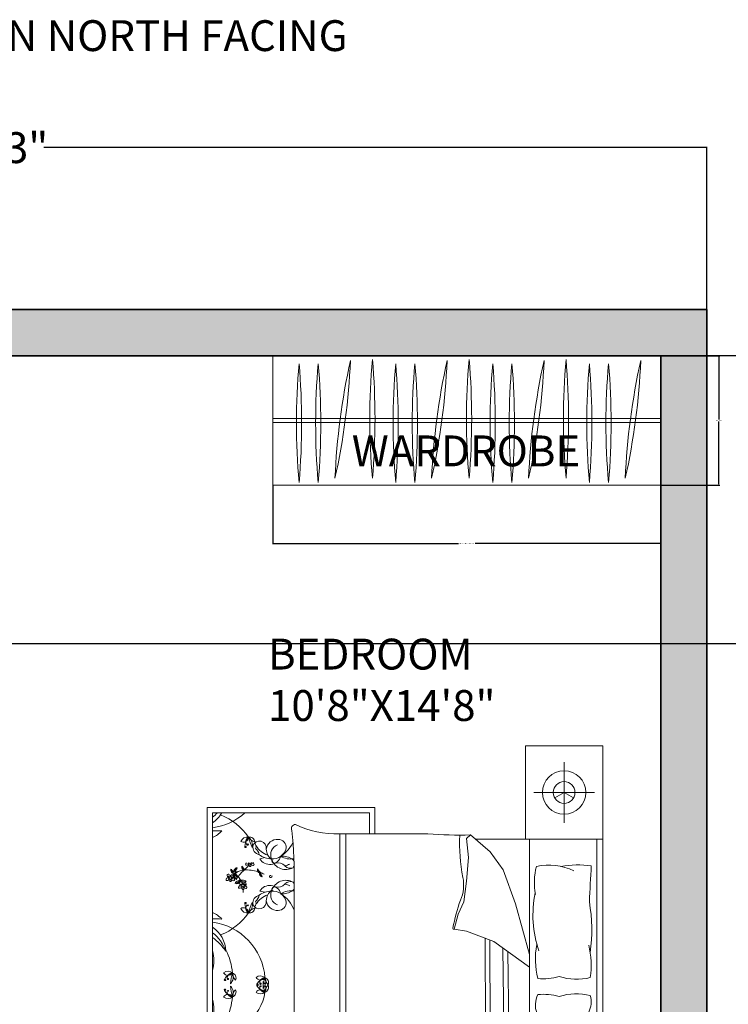
# Model space of a CAD drawing. Units: inches. Extents: x 37 to 706, y -568 to 110.
# Tile 21 of 24: x 224 to 362, y -84 to 108. Entities that reach past the tile are written whole.
import ezdxf

# ---------------------------------------------------------------- set-up
doc = ezdxf.new("R2010")
doc.units = ezdxf.units.IN
doc.header["$MEASUREMENT"] = 0
for name, color, linetype, lineweight in [('A-ANNO-DIMS', 2, 'Continuous', 18), ('A-ANNO-TEXT', 7, 'Continuous', 18), ('A-AREA-IDEN', 7, 'Continuous', 18), ('A-FLOR-CASE', 9, 'Continuous', 18), ('A-FURN', 8, 'Continuous', 13), ('A-WALL', 7, 'Continuous', 35), ('A-WALL-PATT', 252, 'Continuous', 13)]:
    doc.layers.add(name, color=color, linetype=linetype, lineweight=lineweight)
doc.styles.get("Standard").update_dxf_attribs({"font": 'arial.ttf'})
doc.dimstyles.get("Standard").update_dxf_attribs({"dimtxt": 0.18, "dimasz": 0.18, "dimexe": 0.18, "dimexo": 0.0625, "dimgap": 0.09, "dimtad": 0, "dimtih": 1, "dimtoh": 1, "dimdec": 0, "dimzin": 0, "dimdsep": 46, "dimlunit": 3, "dimtxsty": 'Standard', "dimcen": 0.09, "dimadec": 0, "dimazin": 0, "dimtfac": 1, "dimtdec": 0, "dimtofl": 0, "dimtmove": 0, "dimatfit": 3, "dimfxl": 1, "dimtolj": 1, "dimtzin": 0, "dimarcsym": 0})

# ---------------------------------------------------------------- blocks, each defined once
blk = doc.blocks.new('*D2')
at = {"layer": 'A-ANNO-DIMS', "color": 0, "lineweight": -2, "transparency": 16777216}
for p, q in [((78.96, 51.35), (78.96, 82.95)), ((79.14, 82.77), (208.01, 82.77)), ((357.78, 82.77), (228.91, 82.77)), ((357.96, 51.35), (357.96, 82.95))]:
    blk.add_line(p, q, dxfattribs=at)
at = {"layer": 'A-ANNO-DIMS', "color": 0, "transparency": 16777216}
for points in [[(79.14, 82.8), (79.14, 82.74), (78.96, 82.77)], [(357.78, 82.8), (357.78, 82.74), (357.96, 82.77)]]:
    blk.add_solid(points, dxfattribs=at)
at = {"layer": 'Defpoints', "color": 0, "transparency": 16777216}
for p in [(357.96, 82.77), (78.96, 51.29), (357.96, 51.29)]:
    blk.add_point(p, dxfattribs=at)
at = {"layer": 'A-ANNO-DIMS', "color": 0, "transparency": 16777216, "insert": (218.46, 82.77), "char_height": 6, "attachment_point": 5}
blk.add_mtext('\\A1;23\'-3"', dxfattribs=at)
blk = doc.blocks.new('WARDROBE-DOUBLE')
for p, q in [((75.49, 25.16), (0, 25.16)), ((0, 25.16), (0, 0)), ((75.49, 25.16), (75.49, 0)), ((75.49, 13), (0, 13)), ((75.49, 12.16), (0, 12.16)), ((75.49, 0), (0, 0))]:
    blk.add_line(p, q)
for centre, start, end in [((137.01, 12.08), 175.0028, 184.9972), ((-126.78, 12.08), 355.0028, 4.9972), ((140.74, 12.08), 175.0028, 184.9972), ((-123.05, 12.08), 355.0028, 4.9972), ((-117.16, 29.99), 347.508, 357.5023), ((144.38, -4.42), 167.508, 177.5023), ((151.29, 12.89), 175.0028, 184.9972), ((-112.5, 12.89), 355.0028, 4.9972), ((155.82, 12.08), 175.0028, 184.9972), ((-107.97, 12.08), 355.0028, 4.9972), ((159.55, 12.08), 175.0028, 184.9972), ((-104.24, 12.08), 355.0028, 4.9972), ((-98.35, 29.99), 347.508, 357.5023), ((163.19, -4.42), 167.508, 177.5023), ((170.1, 12.89), 175.0028, 184.9972), ((-93.69, 12.89), 355.0028, 4.9972), ((174.7, 12.08), 175.0028, 184.9972), ((-89.09, 12.08), 355.0028, 4.9972), ((178.43, 12.08), 175.0028, 184.9972), ((-85.36, 12.08), 355.0028, 4.9972), ((182.06, -4.42), 167.508, 177.5023), ((-79.47, 29.99), 347.508, 357.5023), ((188.97, 12.89), 175.0028, 184.9972), ((-74.82, 12.89), 355.0028, 4.9972), ((193.51, 12.08), 175.0028, 184.9972), ((-70.28, 12.08), 355.0028, 4.9972), ((197.24, 12.08), 175.0028, 184.9972), ((-66.55, 12.08), 355.0028, 4.9972), ((200.87, -4.42), 167.508, 177.5023), ((-60.66, 29.99), 347.508, 357.5023)]:
    blk.add_arc(centre, 132.4, start, end)
blk = doc.blocks.new('BED-DOUBLE-WITH-NIGHTSTANDS')
for p, q in [((77.02, 90.57), (77.02, 0)), ((69.47, 75.59), (69.47, 87.43)), ((63.56, 81.51), (75.39, 81.51)), ((0, 78.61), (32.62, 78.61)), ((0, 12.59), (0, 78.61)), ((32.62, 78.61), (32.62, 73.49)), ((1.05, 77.56), (1.05, 13.64)), ((31.58, 77.56), (1.05, 77.56)), ((31.58, 73.49), (31.58, 77.56)), ((25.85, 17.62), (25.85, 73.5)), ((26.98, 17.7), (26.98, 73.5)), ((50.48, 72.53), (51.22, 73.26)), ((51.22, 73.26), (55.07, 69.96)), ((50.85, 68.86), (50.48, 72.53)), ((77.02, 72.45), (52.16, 72.45)), ((62.71, 72.45), (62.71, 18.11)), ((75.86, 18.11), (75.86, 72.45)), ((55.07, 69.96), (57.63, 66.48)), ((10.23, 68.64), (11.25, 68.84)), ((50.48, 64.28), (50.85, 68.86)), ((57.63, 66.48), (60.02, 59.87)), ((16.95, 26.9), (16.95, 63.67)), ((49.93, 60.24), (50.48, 64.28)), ((10.23, 62.31), (11.25, 62.11)), ((48.83, 57.86), (49.93, 60.24)), ((60.02, 59.87), (62.71, 50)), ((48.1, 54.92), (48.83, 57.86)), ((50.48, 54.55), (48.1, 54.92)), ((55.8, 52.54), (50.48, 54.55)), ((54.24, 18.43), (54.09, 53.18)), ((55.17, 18.44), (55.03, 52.83)), ((62.71, 47.57), (55.8, 52.54)), ((58.02, 18.39), (57.55, 51.28)), ((58.95, 18.36), (58.49, 50.6)), ((10.23, 28.89), (11.25, 29.09)), ((10.23, 22.56), (11.25, 22.36)), ((31.58, 13.64), (31.58, 17.63)), ((32.62, 17.61), (32.62, 12.59)), ((1.05, 13.64), (31.58, 13.64)), ((69.47, 14.97), (69.47, 3.14)), ((32.62, 12.59), (0, 12.59))]:
    blk.add_line(p, q)
for points in [[(61.93, 72.45), (61.93, 90.57), (77.02, 90.57)], [(69.47, 81.51), (67.64, 80.45)], [(69.47, 81.51), (71.3, 80.45)], [(77.02, 18.11), (61.93, 18.11), (61.93, 0), (77.02, 0)], [(69.47, 9.06), (67.64, 10.11)], [(69.47, 9.06), (71.3, 10.11)]]:
    blk.add_lwpolyline(points)
for points in [[(42.92, 73.45, 0.001242), (25.74, 73.5, -0.127202), (17.18, 75.31)], [(74.76, 67.25, 0.074897), (68.85, 67.14, -0.472817)], [(68.52, 45.71, 0.14099), (74.55, 45.53, 0.235245)], [(68.52, 41.84, -0.14099), (74.55, 42.02, -0.235245)], [(74.76, 23.32, -0.074897), (68.85, 23.42, 0.472817)], [(27.69, 17.73, 0.056112), (22.71, 17.07, 0.095341), (17.91, 15.8)]]:
    blk.add_lwpolyline(points, format="xyb")
for centre, radius in [((69.47, 81.51), 4.23), ((69.47, 81.51), 2.11), ((4.52, 64.91), 0.231), ((6.95, 63.41), 0.231), ((6.95, 27.79), 0.231), ((4.52, 26.28), 0.231), ((69.47, 9.06), 4.23), ((69.47, 9.06), 2.11)]:
    blk.add_circle(centre, radius)
for centre, radius, start, end in [((-3.2, 82.51), 7.18, 306.3036, 316.4814), ((-2.13, 80.43), 5.76, 303.4617, 330.1116), ((-0.54, 86.37), 11.83, 277.745, 311.8856), ((-1.71, 66.13), 11.83, 34.3865, 68.5908), ((17.23, 74.48), 0.836, 93.98, 207.3412), ((-0.79, 77.21), 4.81, 292.5547, 318.9546), ((1.79, 90.38), 16.36, 267.4081, 273.6519), ((7.77, 71.53), 1.31, 77.7115, 159.0387), ((7.06, 72.84), 0.988, 238.4633, 358.2869), ((10.3, 70.85), 2.99, 138.8402, 177.9352), ((8.5, 71.96), 0.967, 117.6827, 223.7762), ((8.28, 71.86), 0.98, 2.9516, 103.728), ((16.12, 74.61), 8.27, 192.5173, 207.1824), ((6.95, 71.3), 1.87, 345.4653, 54.2343), ((9.77, 73.87), 2.02, 211.3827, 255.2969), ((-77.32, 64.75), 94.28, 359.3433, 5.6887), ((48.97, 156.3), 83.07, 265.8294, 271.553), ((83.29, 71.71), 34.18, 177.4519, 191.3392), ((7.46, 70.95), 0.147, 177.9352, 11.4834), ((7.53, 70.96), 0.0713, 11.4834, 127.9409), ((7.89, 71.38), 0.128, 223.7762, 159.7183), ((10.16, 70.71), 1.36, 350.264, 160.8688), ((10.57, 71.04), 1.7, 175.969, 254.3045), ((8.69, 70.99), 0.833, 333.9755, 53.2681), ((13.15, 73.4), 4.28, 211.2614, 251.7045), ((13.65, 70.21), 2.16, 84.9449, 172.8857), ((14.47, 69.36), 2.1, 111.5819, 201.4221), ((13.86, 70.84), 1.53, 354.4856, 91.0538), ((10.57, 74.83), 6.85, 303.6671, 333.2997), ((8.31, 69.21), 1.81, 6.1662, 51.5825), ((12.81, 73.44), 4.86, 236.2883, 266.5076), ((12.18, 69.76), 2.25, 209.9085, 343.1337), ((14.13, 70.59), 2.63, 182.3591, 234.0401), ((12.73, 71.31), 2.72, 265.2933, 346.921), ((16.28, 72.32), 3.75, 238.8218, 279.1554), ((14.65, 65.65), 3.49, 55.785, 94.7304), ((9.29, 67.11), 2.55, 178.3264, 187.1302), ((6.53, 66.75), 0.476, 11.3256, 64.4621), ((8.15, 67.44), 1.43, 190.2588, 210.656), ((1.34, 72.69), 8.6, 313.1541, 322.0459), ((7.66, 67.53), 0.177, 142.4737, 265.053), ((7.89, 67.56), 0.381, 127.7621, 169.0403), ((7.69, 67.89), 0.536, 265.053, 338.3618), ((8.4, 67.15), 0.7, 113.4276, 137.6104), ((8.32, 67.88), 0.231, 183.2768, 356.7232), ((8.49, 67.46), 0.377, 139.7889, 227.6792), ((8.37, 67.33), 0.199, 227.6792, 350.3487), ((7.6, 67.46), 0.755, 353.0852, 15.7171), ((8.1, 67.37), 0.477, 350.3487, 43.6538), ((8.98, 67.87), 0.555, 198.7263, 262.5032), ((8.54, 67.61), 0.22, 1.1081, 91.8675), ((8.68, 67.56), 0.385, 11.5637, 52.6358), ((8.95, 67.49), 0.178, 255.2356, 54.9248), ((13.13, 68.34), 0.562, 167.3041, 285.1471), ((14.65, 65.65), 3.49, 122.7011, 126.3445), ((15.31, 69.41), 2.89, 199.2822, 299.1751), ((13.76, 66), 1.86, 41.5653, 105.1471), ((14.78, 69.85), 2.6, 277.436, 299.9149), ((16.16, 68.13), 1.36, 221.5653, 293.8354), ((15.95, 67.67), 1.09, 30.0293, 52.325), ((15.95, 67.67), 1.09, 314.4517, 333.558), ((75.82, 64.02), 12.14, 165.1039, 191.0369), ((66.47, 55.71), 11.67, 65.1316, 101.7583), ((936.66, 17.33), 863.34, 176.68521, 177.14978), ((4.34, 65.38), 0.455, 157.4086, 261.4386), ((4.09, 65.4), 0.229, 58.0499, 135.6268), ((4.32, 65.26), 0.153, 172.906, 277.132), ((3.82, 64.98), 0.727, 14.7558, 58.0499), ((4.84, 65.17), 0.315, 36.1046, 181.4281), ((4.85, 66.4), 0.258, 124.3538, 214.3923), ((5.23, 66.36), 0.6, 190.3057, 287.1958), ((4.66, 65.42), 0.317, 270.0645, 331.1507), ((5.41, 66.58), 0.697, 176.9701, 248.2913), ((10.38, 70.25), 6.74, 212.6784, 216.3746), ((4.92, 65.2), 0.226, 263.7526, 41.7054), ((5.17, 66.41), 0.267, 216.3746, 291.7548), ((7.53, 62.67), 3.76, 124.0033, 132.4917), ((3.66, 62.2), 4.02, 63.7819, 68.2913), ((5.81, 65.29), 0.639, 128.3208, 208.8162), ((5.81, 66.23), 0.6, 122.8155, 187.3992), ((5.34, 65.98), 0.201, 289.3605, 111.7548), ((5.49, 65.98), 0.201, 221.8703, 44.2646), ((6.41, 65.39), 1.05, 157.2305, 229.0635), ((6.07, 66.15), 0.697, 109.4799, 177.6828), ((6.05, 65.74), 0.619, 174.4544, 220.6188), ((2.53, 62.29), 4.51, 30.544, 49.818), ((5.7, 66.59), 0.258, 56.8636, 146.9021), ((5.83, 66.31), 0.267, 148.8844, 224.2646), ((5.02, 64.86), 0.744, 340.0041, 40.6188), ((11.37, 62.96), 6.74, 145.1882, 148.8844), ((7.53, 62.67), 3.76, 94.756, 119.2041), ((15.54, 57.26), 12.37, 132.2412, 142.1744), ((7.19, 66.85), 0.435, 188.3432, 274.2869), ((7.57, 67.09), 0.759, 210.656, 242.6341), ((8.14, 67.75), 1.46, 218.2101, 226.3071), ((7.07, 66.52), 0.185, 325.7657, 67.4417), ((7.72, 58.94), 7.5, 73.5842, 93.8277), ((12.34, 66.57), 2.55, 178.3264, 187.1302), ((9.58, 66.21), 0.476, 11.3256, 64.4621), ((11.19, 66.9), 1.43, 190.2588, 210.656), ((10.23, 66.31), 0.435, 188.3432, 274.2869), ((10.61, 66.55), 0.759, 210.656, 242.6341), ((11.19, 67.21), 1.46, 218.2101, 226.3071), ((10.11, 65.98), 0.185, 325.7657, 67.4417), ((10.63, 65.65), 0.435, 147.5332, 233.4768), ((11.02, 65.87), 0.759, 179.1859, 211.164), ((10.28, 65.7), 0.185, 354.3784, 96.0543), ((7.72, 58.94), 7.5, 63.0032, 69.8941), ((11.6, 66.22), 1.43, 211.164, 231.5612), ((11.85, 67.38), 2.55, 234.6898, 243.4936), ((11.87, 66.07), 1.46, 195.5129, 203.6099), ((10.23, 65.12), 0.476, 357.3579, 50.4944), ((12.28, 65.21), 0.175, 12.7051, 190.4384), ((12.38, 65.23), 0.284, 190.4384, 10.4136), ((3.86, 64.56), 0.177, 142.4737, 265.053), ((4.09, 64.6), 0.381, 61.2196, 169.0403), ((3.89, 64.92), 0.536, 265.053, 338.3618), ((4.6, 64.19), 0.7, 113.4276, 137.6104), ((4.69, 64.5), 0.377, 139.7889, 227.6792), ((4.57, 64.37), 0.199, 227.6792, 350.3487), ((3.8, 64.5), 0.755, 353.0852, 15.7171), ((4.29, 64.41), 0.477, 350.3487, 43.6538), ((5.18, 64.9), 0.555, 198.7263, 262.5032), ((4.93, 65.34), 0.363, 221.8413, 265.7877), ((4.74, 64.65), 0.22, 1.1081, 91.8675), ((4.88, 64.6), 0.385, 11.5637, 86.365), ((5.15, 64.53), 0.178, 255.2356, 54.9248), ((5.92, 65.34), 0.764, 207.7043, 254.3516), ((5.43, 64.9), 1.05, 270.278, 342.111), ((6.13, 63.58), 0.744, 98.7227, 159.3375), ((5.75, 64.54), 0.764, 244.9899, 291.6373), ((5.92, 64.93), 0.619, 278.7227, 324.8872), ((5.81, 64.43), 0.639, 290.5253, 358.5375), ((6.52, 63.09), 0.381, 61.2196, 169.0403), ((6.32, 63.41), 0.536, 265.053, 338.3618), ((6.77, 63.88), 0.455, 157.4086, 261.4386), ((6.52, 63.89), 0.229, 58.0499, 135.6268), ((7.06, 64.61), 0.639, 182.8499, 266.1226), ((6.81, 65.06), 0.619, 231.7607, 277.9252), ((7.29, 65.17), 1.05, 214.5369, 286.3699), ((7.03, 62.68), 0.7, 113.4276, 137.6104), ((6.76, 63.75), 0.153, 172.906, 277.132), ((6.25, 63.47), 0.727, 14.7558, 58.0499), ((2.53, 62.29), 4.51, 23.0501, 23.8477), ((7.12, 62.99), 0.377, 139.7889, 227.6792), ((7, 63.71), 0.744, 37.3105, 97.9252), ((7.27, 63.66), 0.315, 36.1046, 181.4281), ((6.23, 62.99), 0.755, 353.0852, 15.7171), ((7.08, 64.73), 0.764, 265.0106, 311.658), ((6.72, 62.9), 0.477, 350.3487, 43.6538), ((7.61, 63.4), 0.555, 198.7263, 262.5032), ((7.09, 63.91), 0.317, 270.0645, 331.1507), ((7.36, 63.83), 0.363, 221.8413, 265.7877), ((7.17, 63.14), 0.22, 1.1081, 91.8675), ((7.36, 63.7), 0.226, 263.7526, 41.7054), ((7.31, 63.09), 0.385, 11.5637, 86.365), ((12.18, 61.19), 2.25, 16.8663, 150.0915), ((15.31, 61.54), 2.89, 60.8249, 160.7178), ((13.76, 64.95), 1.86, 254.8529, 318.4347), ((14.78, 61.1), 2.6, 60.0851, 82.564), ((16.16, 62.82), 1.36, 66.1646, 138.4347), ((15.95, 63.28), 1.09, 23.229, 45.5483), ((42.55, 63.54), 7.37, 336.2616, 11.3392), ((6.29, 63.06), 0.177, 142.4737, 265.053), ((7, 62.86), 0.199, 227.6792, 350.3487), ((2.53, 62.29), 4.51, 357.1071, 4.7585), ((7.58, 63.02), 0.178, 255.2356, 54.9248), ((10.57, 59.91), 1.7, 105.6955, 184.031), ((8.31, 61.74), 1.81, 308.4175, 353.8338), ((13.15, 57.54), 4.28, 108.2955, 148.7386), ((12.81, 57.5), 4.86, 93.4924, 123.7117), ((14.13, 60.36), 2.63, 125.9599, 177.6409), ((14.47, 61.59), 2.1, 158.5779, 248.4181), ((12.73, 59.64), 2.72, 13.079, 94.7067), ((13.13, 62.61), 0.562, 74.8529, 192.6959), ((14.65, 65.3), 3.49, 233.6555, 237.2989), ((16.28, 58.63), 3.75, 79.7133, 121.1782), ((14.65, 65.3), 3.49, 265.2696, 304.215), ((10.57, 56.11), 6.85, 21.4941, 56.3329), ((15.95, 63.28), 1.09, 307.675, 336.7144), ((84.45, 57.63), 21.05, 168.0397, 199.2615), ((7.46, 60), 0.147, 348.5166, 182.0648), ((10.3, 60.1), 2.99, 182.0648, 221.1598), ((7.53, 59.98), 0.0713, 232.0591, 348.5166), ((8.5, 58.99), 0.967, 136.2238, 242.3173), ((7.94, 59.56), 0.0771, 200.2667, 136.2271), ((6.95, 59.65), 1.87, 305.7657, 14.5347), ((16.12, 56.34), 8.27, 152.8176, 167.4827), ((10.16, 60.24), 1.36, 199.1312, 9.736), ((8.69, 59.96), 0.833, 306.7319, 26.0245), ((13.65, 60.74), 2.16, 187.1143, 275.0551), ((13.86, 60.11), 1.53, 268.9462, 5.5144), ((82.33, 48.63), 35.12, 160.1194, 169.3383), ((41.99, 54.84), 32.85, 352.2196, 9.497), ((-0.79, 53.74), 4.81, 41.0454, 67.4453), ((-1.71, 64.81), 11.83, 291.4092, 325.6135), ((7.06, 58.1), 0.988, 1.7131, 121.5367), ((7.77, 59.41), 1.31, 200.9613, 282.2885), ((8.28, 59.09), 0.98, 256.272, 357.0484), ((9.77, 57.08), 2.02, 104.7031, 148.6173), ((1.79, 40.57), 16.36, 86.3481, 92.5919), ((-0.54, 44.58), 11.83, 4.4623, 82.255), ((-2.13, 50.51), 5.76, 1.272, 56.5383), ((-3.2, 48.44), 7.18, 17.8504, 53.6964), ((48.03, 55.13), 0.219, 178.8623, 289.7536), ((-5.22, 44.66), 10.68, 34.0123, 54.053), ((79.85, 49.11), 15.97, 169.8617, 193.6238), ((58.59, 47.9), 16.14, 351.5249, 13.96), ((-5.17, 48.79), 6.5, 343.5431, 17.0202), ((-6.88, 45.48), 11.83, 4.4623, 27.4146), ((-8.52, 46.22), 9.62, 4.3787, 5.6357), ((-15.11, 41.15), 17.18, 19.7217, 19.9028), ((4.03, 45.43), 1.31, 47.7873, 129.1145), ((4.07, 46.92), 0.988, 208.5391, 328.3627), ((5.88, 43.58), 2.99, 108.9159, 148.011), ((4.87, 45.44), 0.967, 87.7585, 193.852), ((12.81, 43.93), 8.27, 162.593, 177.2582), ((3.21, 45.64), 1.87, 315.5411, 24.3101), ((6.93, 46.46), 2.02, 181.4585, 225.3727), ((4.64, 45.46), 0.98, 333.0274, 73.8037), ((3.47, 45.08), 0.147, 148.011, 341.5592), ((3.54, 45.06), 0.0713, 341.5592, 98.0167), ((4.06, 45.24), 0.128, 193.852, 129.9245), ((10.37, 44.53), 1.31, 47.7873, 129.1145), ((10.41, 46.02), 0.988, 208.5391, 328.3627), ((9.8, 44.18), 0.147, 148.011, 341.5592), ((9.8, 44), 0.147, 18.4408, 211.989), ((12.22, 42.67), 2.99, 108.9159, 148.011), ((9.88, 44.15), 0.0713, 341.5592, 98.0167), ((9.88, 44.03), 0.0713, 261.9833, 18.4408), ((11.21, 44.53), 0.967, 87.7585, 193.852), ((10.39, 44.33), 0.128, 193.852, 129.9245), ((9.54, 44.73), 1.87, 315.5411, 24.3101), ((19.14, 43.02), 8.27, 162.593, 177.2582), ((9.54, 43.45), 1.87, 335.6899, 44.4589), ((19.14, 45.16), 8.27, 182.7418, 197.407), ((10.97, 44.56), 0.98, 333.0274, 73.8037), ((13.27, 45.55), 2.02, 181.4585, 225.3727), ((10.97, 43.62), 0.98, 286.1963, 26.9726), ((13.27, 42.63), 2.02, 134.6273, 178.5415), ((65.49, 56.38), 11.1, 264.0129, 285.8293), ((2.19, 43.98), 9.15, 262.8636, 351.8197), ((4.07, 41.26), 0.988, 31.6373, 151.4609), ((3.47, 43.1), 0.147, 18.4408, 211.989), ((5.88, 44.6), 2.99, 211.989, 251.0841), ((3.54, 43.12), 0.0713, 261.9833, 18.4408), ((4.87, 42.74), 0.967, 166.148, 272.2415), ((4.11, 42.95), 0.0771, 230.1909, 166.0209), ((12.81, 44.25), 8.27, 182.7418, 197.407), ((3.21, 42.54), 1.87, 335.6899, 44.4589), ((6.93, 41.72), 2.02, 134.6273, 178.5415), ((4.64, 42.72), 0.98, 286.1963, 26.9726), ((10.41, 42.16), 0.988, 31.6373, 151.4609), ((10.37, 43.65), 1.31, 230.8855, 312.2127), ((12.22, 45.51), 2.99, 211.989, 251.0841), ((11.21, 43.65), 0.967, 166.148, 272.2415), ((10.44, 43.86), 0.0771, 230.1909, 166.0209), ((68.68, 40.17), 4.8, 155.0183, 198.5407), ((65.49, 31.16), 11.1, 74.1707, 95.9871), ((-5.17, 39.39), 6.5, 342.9798, 16.4569), ((-8.52, 41.96), 9.62, 354.3643, 355.6213), ((-15.11, 47.03), 17.18, 340.0972, 340.2783), ((4.03, 42.75), 1.31, 230.8855, 312.2127), ((-6.88, 42.69), 11.83, 332.5854, 355.5377), ((70.25, 40.78), 4.48, 333.3437, 16.1026), ((3.02, 42.8), 5.3, 248.117, 276.6195), ((1.55, 37.94), 2.12, 256.3898, 349.0739), ((1.84, 39.54), 2.68, 252.8609, 311.9049), ((-1.71, 26.39), 11.83, 34.3865, 68.5908), ((74.93, 31.78), 11.53, 153.8761, 196.1746), ((58.92, 34.06), 15.92, 346.3427, 11.1841), ((1.79, 50.63), 16.36, 267.4081, 273.6519), ((-0.79, 37.46), 4.81, 292.5547, 318.9546), ((7.77, 31.78), 1.31, 77.7115, 159.0387), ((7.06, 33.09), 0.988, 238.4633, 358.2869), ((10.3, 31.1), 2.99, 138.8402, 177.9352), ((8.5, 32.21), 0.967, 117.6827, 223.7762), ((8.28, 32.11), 0.98, 2.9516, 103.728), ((9.77, 34.12), 2.02, 211.3827, 255.2969), ((6.95, 31.55), 1.87, 345.4653, 54.2343), ((16.12, 34.86), 8.27, 192.5173, 207.1824), ((13.65, 30.46), 2.16, 84.9449, 172.8857), ((13.86, 31.09), 1.53, 354.4856, 91.0538), ((10.57, 35.08), 6.85, 303.6671, 338.5059), ((7.46, 31.2), 0.147, 177.9352, 11.4834), ((7.53, 31.21), 0.0713, 11.4834, 127.9409), ((7.89, 31.63), 0.128, 223.7762, 159.7183), ((10.16, 30.96), 1.36, 350.264, 160.8688), ((10.57, 31.29), 1.7, 175.969, 254.3045), ((8.69, 31.24), 0.833, 333.9755, 53.2681), ((8.31, 29.46), 1.81, 6.1662, 51.5825), ((13.15, 33.66), 4.28, 211.2614, 251.7045), ((14.13, 30.84), 2.63, 182.3591, 234.0401), ((14.47, 29.61), 2.1, 111.5819, 201.4221), ((12.73, 31.56), 2.72, 265.2933, 346.921), ((2.53, 28.91), 4.51, 355.2415, 2.8929), ((12.81, 33.7), 4.86, 236.2883, 266.5076), ((12.18, 30.01), 2.25, 209.9085, 343.1337), ((14.65, 25.9), 3.49, 122.7011, 126.3445), ((16.28, 32.57), 3.75, 238.8218, 280.2867), ((14.65, 25.9), 3.49, 55.785, 94.7304), ((15.95, 27.92), 1.09, 23.2856, 52.325), ((75.82, 26.55), 12.14, 168.9631, 194.8961), ((936.66, 73.23), 863.34, 182.85022, 183.31479), ((3.86, 26.63), 0.177, 94.947, 217.5263), ((3.89, 26.28), 0.536, 21.6382, 94.947), ((4.69, 26.7), 0.377, 132.3208, 220.2111), ((4.57, 26.83), 0.199, 9.6513, 132.3208), ((4.29, 26.79), 0.477, 316.3462, 9.6513), ((5.18, 26.29), 0.555, 97.4968, 161.2737), ((5.15, 26.67), 0.178, 305.0752, 104.7644), ((5.75, 26.66), 0.764, 68.3627, 115.0101), ((5.43, 26.3), 1.05, 17.889, 89.722), ((6.13, 27.61), 0.744, 200.6625, 261.2773), ((5.92, 26.27), 0.619, 35.1128, 81.2773), ((5.81, 26.77), 0.639, 1.4625, 69.4747), ((6.29, 28.14), 0.177, 94.947, 217.5263), ((6.52, 28.11), 0.381, 190.9597, 298.7804), ((6.32, 27.78), 0.536, 21.6382, 94.947), ((6.77, 27.32), 0.455, 98.5614, 202.5914), ((6.52, 27.31), 0.229, 224.3732, 301.9501), ((7.06, 26.59), 0.639, 93.8774, 177.1501), ((7.29, 26.03), 1.05, 73.6301, 145.4631), ((7.03, 28.52), 0.7, 222.3896, 246.5724), ((6.76, 27.45), 0.153, 82.868, 187.094), ((6.25, 27.73), 0.727, 301.9501, 345.2442), ((2.53, 28.91), 4.51, 336.1523, 336.9499), ((7.12, 28.21), 0.377, 132.3208, 220.2111), ((7, 28.34), 0.199, 9.6513, 132.3208), ((7, 27.49), 0.744, 262.0748, 322.6895), ((6.23, 28.2), 0.755, 344.2829, 6.9148), ((7.27, 27.54), 0.315, 178.5719, 323.8954), ((7.08, 26.46), 0.764, 48.342, 94.9894), ((6.72, 28.3), 0.477, 316.3462, 9.6513), ((7.61, 27.8), 0.555, 97.4968, 161.2737), ((7.36, 27.37), 0.363, 94.2123, 138.1587), ((7.09, 27.29), 0.317, 28.8493, 89.9355), ((7.17, 28.06), 0.22, 268.1325, 358.8919), ((7.31, 28.11), 0.385, 273.635, 348.4363), ((7.36, 27.5), 0.226, 318.2946, 96.2474), ((7.58, 28.18), 0.178, 305.0752, 104.7644), ((13.13, 28.59), 0.562, 167.3041, 285.1471), ((15.31, 29.66), 2.89, 199.2822, 299.1751), ((13.76, 26.25), 1.86, 41.5653, 105.1471), ((14.78, 30.1), 2.6, 277.436, 299.9149), ((16.16, 28.38), 1.36, 221.5653, 293.8354), ((-71.13, 24.12), 88.13, 355.2402, 1.8035), ((15.95, 27.92), 1.09, 314.4517, 336.7144), ((4.09, 26.6), 0.381, 190.9597, 298.7804), ((4.34, 25.81), 0.455, 98.5614, 202.5914), ((4.09, 25.8), 0.229, 224.3732, 301.9501), ((4.6, 27.01), 0.7, 222.3896, 246.5724), ((4.32, 25.94), 0.153, 82.868, 187.094), ((3.82, 26.22), 0.727, 301.9501, 345.2442), ((4.84, 26.03), 0.315, 178.5719, 323.8954), ((3.8, 26.7), 0.755, 344.2829, 6.9148), ((4.85, 24.8), 0.258, 145.6077, 235.6462), ((5.23, 24.83), 0.6, 72.8042, 169.6943), ((4.93, 25.86), 0.363, 94.2123, 138.1587), ((4.66, 25.78), 0.317, 28.8493, 89.9355), ((5.41, 24.62), 0.697, 111.7087, 183.0299), ((10.38, 20.95), 6.74, 143.6254, 147.3216), ((4.74, 26.55), 0.22, 268.1325, 358.8919), ((4.88, 26.6), 0.385, 273.635, 348.4363), ((4.92, 25.99), 0.226, 318.2946, 96.2474), ((5.17, 24.78), 0.267, 68.2452, 143.6254), ((7.53, 28.53), 3.76, 227.5083, 235.9967), ((3.66, 29), 4.02, 291.7087, 296.2181), ((5.81, 25.91), 0.639, 151.1838, 231.6792), ((5.81, 24.97), 0.6, 172.6008, 237.1845), ((5.92, 25.86), 0.764, 105.6484, 152.2957), ((5.34, 25.22), 0.201, 248.2452, 70.6395), ((6.41, 25.8), 1.05, 130.9365, 202.7695), ((5.49, 25.22), 0.201, 315.7354, 138.1297), ((6.07, 25.05), 0.697, 182.3172, 250.5201), ((6.05, 25.46), 0.619, 139.3812, 185.5456), ((2.53, 28.91), 4.51, 310.182, 329.456), ((5.83, 24.89), 0.267, 135.7354, 211.1156), ((5.02, 26.34), 0.744, 319.3812, 19.9959), ((7.53, 28.53), 3.76, 240.7959, 265.244), ((15.54, 33.94), 12.37, 217.8256, 227.7588), ((6.81, 26.14), 0.619, 82.0748, 128.2393), ((7.72, 32.26), 7.5, 266.1723, 286.4158), ((11.19, 24.3), 1.43, 149.344, 169.7412), ((12.34, 24.63), 2.55, 172.8698, 181.6736), ((10.23, 24.88), 0.435, 85.7131, 171.6568), ((10.61, 24.64), 0.759, 117.3659, 149.344), ((11.19, 23.99), 1.46, 133.6929, 141.7899), ((10.11, 25.21), 0.185, 292.5583, 34.2343), ((10.63, 25.55), 0.435, 126.5232, 212.4668), ((11.02, 25.33), 0.759, 148.836, 180.8141), ((10.28, 25.5), 0.185, 263.9457, 5.6216), ((7.72, 32.26), 7.5, 290.1059, 296.9968), ((11.6, 24.98), 1.43, 128.4388, 148.836), ((11.85, 23.82), 2.55, 116.5064, 125.3102), ((11.87, 25.13), 1.46, 156.3901, 164.4871), ((10.23, 26.08), 0.476, 309.5056, 2.6421), ((12.28, 25.98), 0.175, 169.5616, 347.2949), ((12.38, 25.96), 0.284, 349.5864, 169.5616), ((5.7, 24.61), 0.258, 213.0979, 303.1364), ((11.37, 28.24), 6.74, 211.1156, 214.8118), ((8.15, 23.76), 1.43, 149.344, 169.7412), ((9.29, 24.09), 2.55, 172.8698, 181.6736), ((6.53, 24.45), 0.476, 295.5379, 348.6744), ((7.19, 24.34), 0.435, 85.7131, 171.6568), ((7.57, 24.1), 0.759, 117.3659, 149.344), ((8.14, 23.45), 1.46, 133.6929, 141.7899), ((7.07, 24.67), 0.185, 292.5583, 34.2343), ((1.34, 18.5), 8.6, 37.9541, 46.8459), ((7.66, 23.67), 0.177, 94.947, 217.5263), ((7.89, 23.64), 0.381, 190.9597, 232.2379), ((7.69, 23.31), 0.536, 21.6382, 94.947), ((8.4, 24.05), 0.7, 222.3896, 246.5724), ((8.32, 23.32), 0.231, 3.2768, 176.7232), ((8.49, 23.74), 0.377, 132.3208, 220.2111), ((8.37, 23.87), 0.199, 9.6513, 132.3208), ((7.6, 23.73), 0.755, 344.2829, 6.9148), ((8.1, 23.82), 0.477, 316.3462, 9.6513), ((8.98, 23.33), 0.555, 97.4968, 161.2737), ((8.54, 23.59), 0.22, 268.1325, 358.8919), ((8.95, 23.71), 0.178, 305.0752, 104.7644), ((8.68, 23.64), 0.385, 307.3642, 348.4363), ((9.58, 24.98), 0.476, 295.5379, 348.6744), ((12.18, 21.44), 2.25, 16.8663, 150.0915), ((13.13, 22.86), 0.562, 74.8529, 192.6959), ((15.31, 21.79), 2.89, 60.8249, 160.7178), ((13.76, 25.2), 1.86, 254.8529, 318.4347), ((14.78, 21.35), 2.6, 60.0851, 82.564), ((16.16, 23.07), 1.36, 66.1646, 138.4347), ((15.95, 23.53), 1.09, 307.675, 342.5814), ((15.95, 23.53), 1.09, 16.6343, 45.5483), ((66.47, 34.85), 11.67, 258.2417, 294.8684), ((10.57, 20.16), 1.7, 105.6955, 184.031), ((8.31, 21.99), 1.81, 308.4175, 353.8338), ((13.15, 17.79), 4.28, 108.2955, 148.7386), ((12.81, 17.75), 4.86, 93.4924, 123.7117), ((14.13, 20.61), 2.63, 125.9599, 177.6409), ((14.47, 21.84), 2.1, 158.5779, 248.4181), ((12.73, 19.89), 2.72, 13.079, 94.7067), ((14.65, 25.55), 3.49, 233.6555, 237.2989), ((16.28, 18.88), 3.75, 79.249, 121.1782), ((14.65, 25.55), 3.49, 265.2696, 304.215), ((10.57, 16.37), 6.85, 23.6453, 56.3329), ((7.06, 18.36), 0.988, 1.7131, 121.5367), ((7.77, 19.67), 1.31, 200.9613, 282.2885), ((7.46, 20.25), 0.147, 348.5166, 182.0648), ((10.3, 20.35), 2.99, 182.0648, 221.1598), ((7.53, 20.24), 0.0713, 232.0591, 348.5166), ((8.5, 19.24), 0.967, 136.2238, 242.3173), ((7.94, 19.81), 0.0771, 200.2667, 136.2271), ((16.12, 16.59), 8.27, 152.8176, 167.4827), ((6.95, 19.9), 1.87, 305.7657, 14.5347), ((9.77, 17.33), 2.02, 104.7031, 148.6173), ((8.28, 19.34), 0.98, 256.272, 357.0484), ((10.16, 20.49), 1.36, 199.1312, 9.736), ((8.69, 20.21), 0.833, 306.7319, 26.0245), ((13.65, 20.99), 2.16, 187.1143, 275.0551), ((13.86, 20.36), 1.53, 268.9462, 5.5144), ((-0.79, 13.99), 4.81, 41.0454, 67.4453), ((-1.71, 25.06), 11.83, 291.4092, 325.6135), ((45.72, -193.78), 212.28, 89.1145, 94.8735), ((51.64, -144.24), 162.73, 86.1, 90.9282), ((1.79, 0.82), 16.36, 86.3481, 92.5919), ((-0.54, 4.83), 11.83, 48.1144, 82.255), ((-2.13, 10.76), 5.76, 29.8884, 56.5383), ((17.45, 16.48), 0.826, 156.5219, 303.8264), ((-3.2, 8.69), 7.18, 43.5186, 53.6964)]:
    blk.add_arc(centre, radius, start, end)
blk = doc.blocks.new('*D21')
at = {"layer": 'A-ANNO-DIMS', "color": 0, "lineweight": -2, "transparency": 16777216}
for p, q in [((273.47, 17.07), (273.47, 5.63)), ((348.96, 17.07), (348.96, 5.63)), ((273.65, 5.81), (309.59, 5.81)), ((348.78, 5.81), (312.84, 5.81))]:
    blk.add_line(p, q, dxfattribs=at)
at = {"layer": 'A-ANNO-DIMS', "color": 0, "transparency": 16777216}
for points in [[(273.65, 5.84), (273.65, 5.78), (273.47, 5.81)], [(348.78, 5.84), (348.78, 5.78), (348.96, 5.81)]]:
    blk.add_solid(points, dxfattribs=at)
at = {"layer": 'Defpoints', "color": 0, "transparency": 16777216}
for p in [(273.47, 17.13), (348.96, 17.13), (348.96, 5.81)]:
    blk.add_point(p, dxfattribs=at)
at = {"layer": 'A-ANNO-DIMS', "color": 0, "transparency": 16777216, "insert": (311.21, 5.81), "char_height": 0.18, "attachment_point": 5}
blk.add_mtext('\\A1;WARDROBE 6\'-3 1/2" TYP.', dxfattribs=at)
blk = doc.blocks.new('*D22')
at = {"layer": 'A-ANNO-DIMS', "color": 0, "lineweight": -2, "transparency": 16777216}
for p, q in [((349.02, 42.29), (360.46, 42.29)), ((360.28, 42.11), (360.28, 29.89)), ((360.28, 17.31), (360.28, 29.53)), ((349.02, 17.13), (360.46, 17.13))]:
    blk.add_line(p, q, dxfattribs=at)
at = {"layer": 'A-ANNO-DIMS', "color": 0, "transparency": 16777216}
for points in [[(360.25, 42.11), (360.31, 42.11), (360.28, 42.29)], [(360.25, 17.31), (360.31, 17.31), (360.28, 17.13)]]:
    blk.add_solid(points, dxfattribs=at)
at = {"layer": 'Defpoints', "color": 0, "transparency": 16777216}
for p in [(348.96, 42.29), (360.28, 42.29), (348.96, 17.13)]:
    blk.add_point(p, dxfattribs=at)
at = {"layer": 'A-ANNO-DIMS', "color": 0, "transparency": 16777216, "insert": (360.28, 29.71), "char_height": 0.18, "attachment_point": 5}
blk.add_mtext('\\A1;2\'-1" TYP.', dxfattribs=at)
blk = doc.blocks.new('*D42')
at = {"layer": 'A-ANNO-DIMS', "color": 0, "lineweight": -2, "transparency": 16777216}
for p, q in [((402.9, 42.29), (46.03, 42.29)), ((46.21, 42.11), (46.21, 14.47)), ((46.21, -13.53), (46.21, 14.11)), ((402.9, -13.71), (46.03, -13.71))]:
    blk.add_line(p, q, dxfattribs=at)
at = {"layer": 'A-ANNO-DIMS', "color": 0, "transparency": 16777216}
for points in [[(46.18, 42.11), (46.24, 42.11), (46.21, 42.29)], [(46.18, -13.53), (46.24, -13.53), (46.21, -13.71)]]:
    blk.add_solid(points, dxfattribs=at)
at = {"layer": 'Defpoints', "color": 0, "transparency": 16777216}
for p in [(402.96, 42.29), (46.21, -13.71), (402.96, -13.71)]:
    blk.add_point(p, dxfattribs=at)
at = {"layer": 'A-ANNO-DIMS', "color": 0, "transparency": 16777216, "insert": (46.21, 14.29), "char_height": 0.18, "attachment_point": 5}
blk.add_mtext('\\A1;4\'-8"', dxfattribs=at)

msp = doc.modelspace()

# ---------------------------------------------------------------- hatches: boundary and pattern name
at = {"layer": 'A-WALL-PATT'}
h = msp.add_hatch(color=256, dxfattribs=at)
h.dxf.hatch_style = 1
h.paths.add_polyline_path([(220.96, -351.71), (211.96, -351.71), (211.96, -513.71), (254.96, -513.71), (254.96, -504.71), (220.96, -504.71)], flags=17)
h.paths.add_polyline_path([(220.96, -294.71), (211.96, -294.71), (211.96, -303.71), (220.96, -303.71)], flags=17)
h.paths.add_polyline_path([(175.96, -294.71), (155.87, -294.71), (155.87, -303.71), (155.96, -303.71), (175.96, -303.71)], flags=17)
h.paths.add_polyline_path([(220.96, -16.71), (211.96, -16.71), (211.96, -142.71), (220.96, -142.71)], flags=17)
h.paths.add_polyline_path([(357.96, 51.29), (78.96, 51.29), (78.96, -513.71), (87.96, -513.71), (87.96, -303.71), (95.87, -303.71), (95.87, -294.71), (87.96, -294.71), (87.96, -142.71), (187.96, -142.71), (187.96, -133.71), (87.96, -133.71), (87.96, -25.71), (106.96, -25.71), (106.96, -16.71), (87.96, -16.71), (87.96, 42.29), (348.96, 42.29), (348.96, 17.13), (348.96, -133.71), (246.96, -133.71), (246.96, -142.71), (348.96, -142.71), (348.96, -294.71), (251.96, -294.71), (251.96, -303.71), (348.96, -303.71), (348.96, -351.71), (260.96, -351.71), (260.96, -329.71), (251.96, -329.71), (251.96, -360.71), (327.45, -360.71), (348.96, -360.71), (348.96, -504.71), (314.96, -504.71), (314.96, -513.71), (357.96, -513.71)])
h.paths.add_polyline_path([(416.96, -303.71), (402.96, -303.71), (402.96, -151.71), (478.96, -151.71), (478.96, -142.71), (402.96, -142.71), (402.96, -22.71), (409.96, -22.71), (409.96, -13.71), (402.96, -13.71), (402.96, 42.29), (663.96, 42.29), (663.96, -303.71), (566.96, -303.71), (566.96, -312.71), (663.96, -312.71), (663.96, -360.71), (575.96, -360.71), (575.96, -338.71), (566.96, -338.71), (566.96, -360.71), (566.96, -369.71), (642.45, -369.71), (663.96, -369.71), (663.96, -513.71), (629.96, -513.71), (629.96, -522.71), (672.96, -522.71), (672.96, 51.29), (393.96, 51.29), (393.96, -522.71), (402.96, -522.71), (402.96, -312.71), (416.96, -312.71)])
h.paths.add_polyline_path([(490.96, -303.71), (476.96, -303.71), (476.96, -312.71), (490.96, -312.71)], flags=17)
h.paths.add_polyline_path([(535.96, -303.71), (526.96, -303.71), (526.96, -312.71), (535.96, -312.71)], flags=17)
h.paths.add_polyline_path([(535.96, -369.71), (526.96, -369.71), (526.96, -522.71), (569.96, -522.71), (569.96, -513.71), (535.96, -513.71)], flags=17)
h.paths.add_polyline_path([(511.96, -13.71), (502.96, -13.71), (502.96, -151.71), (511.96, -151.71)], flags=17)
h.paths.add_polyline_path([(651.54, -142.71), (651.54, -120.18), (642.54, -120.18), (642.54, -142.71), (550.54, -142.71), (550.54, -120.71), (541.54, -120.71), (541.54, -142.71), (537.96, -142.71), (537.96, -151.71), (651.54, -151.71)], flags=17)
h.paths.add_polyline_path([(651.54, -85.71), (541.54, -85.71), (541.54, -94.71), (651.54, -94.71)], flags=17)
h.paths.add_polyline_path([(476.96, -13.71), (469.96, -13.71), (469.96, -22.71), (476.96, -22.71)], flags=17)
h.paths.add_polyline_path([(185.96, -16.71), (166.96, -16.71), (166.96, -25.71), (185.96, -25.71)], flags=17)
h.paths.add_polyline_path([(168.91, -414.72), (214.62, -414.72), (214.62, -392.33), (168.91, -392.33)], flags=25)

# ---------------------------------------------------------------- linework, layer by layer
at = {"layer": 'A-WALL'}
for p, q in [((78.96, 51.29), (357.96, 51.29)), ((357.96, 51.29), (357.96, -513.71)), ((87.96, 42.29), (348.96, 42.29)), ((348.96, 42.29), (348.96, -133.71))]:
    msp.add_line(p, q, dxfattribs=at)

# ---------------------------------------------------------------- block references
at = {"layer": 'A-FLOR-CASE'}
msp.add_blockref('WARDROBE-DOUBLE', (273.47, 17.13), dxfattribs=at)
at = {"layer": 'A-FURN'}
msp.add_blockref('BED-DOUBLE-WITH-NIGHTSTANDS', (260.7, -124.14), dxfattribs=at)

# ---------------------------------------------------------------- texts
at = {"layer": 'A-ANNO-TEXT', "insert": (154.79, 107.55), "char_height": 6, "attachment_point": 1}
msp.add_mtext('22X45HOUSE PLAN NORTH FACING', dxfattribs=at)
at = {"layer": 'A-ANNO-TEXT', "insert": (288.85, 26.8), "char_height": 6, "attachment_point": 1}
msp.add_mtext_dynamic_manual_height_columns('WARDROBE', width=0.234, gutter_width=1, heights=[0], dxfattribs=at)
at = {"layer": 'A-AREA-IDEN', "insert": (272.55, -12.72), "char_height": 6, "attachment_point": 1}
msp.add_mtext('BEDROOM\\P10\'8"X14\'8"', dxfattribs=at)

# ---------------------------------------------------------------- dimensions: what is measured, and where the dimension line sits
at = {"layer": 'A-ANNO-DIMS'}
dim = msp.add_linear_dim(base=(357.96, 82.77), p1=(78.96, 51.29), p2=(357.96, 51.29), dimstyle='Standard', override={"dimtxt": 6, "dimclrd": 0, "dimclre": 0, "dimclrt": 0}, dxfattribs=at)
dim.commit()
dim.dimension.update_dxf_attribs({"geometry": '*D2', "text_midpoint": (218.46, 82.77)})
dim = msp.add_linear_dim(base=(46.21, -13.71), p1=(402.96, 42.29), p2=(402.96, -13.71), angle=90, dimstyle='Standard', override={"dimdec": 1, "dimlfac": 1, "dimrnd": 0, "dimzin": 1, "dimdsep": 46, "dimlunit": 4, "dimfrac": 2}, dxfattribs=at)
dim.commit()
dim.dimension.update_dxf_attribs({"geometry": '*D42', "text_midpoint": (46.21, 14.29)})
dim = msp.add_linear_dim(base=(360.28, 42.29), p1=(348.96, 17.13), p2=(348.96, 42.29), angle=90, text='<> TYP.', dimstyle='Standard', override={"dimdec": 1, "dimlfac": 1, "dimrnd": 0, "dimzin": 1, "dimdsep": 46, "dimlunit": 4, "dimfrac": 2}, dxfattribs=at)
dim.commit()
dim.dimension.update_dxf_attribs({"geometry": '*D22', "text_midpoint": (360.28, 29.71)})
dim = msp.add_linear_dim(base=(348.96, 5.81), p1=(273.47, 17.13), p2=(348.96, 17.13), text='WARDROBE <> TYP.', dimstyle='Standard', override={"dimdec": 1, "dimlfac": 1, "dimrnd": 0, "dimzin": 1, "dimdsep": 46, "dimlunit": 4, "dimfrac": 2}, dxfattribs=at)
dim.commit()
dim.dimension.update_dxf_attribs({"geometry": '*D21', "text_midpoint": (311.21, 5.81)})

doc.saveas('drawing.dxf')
